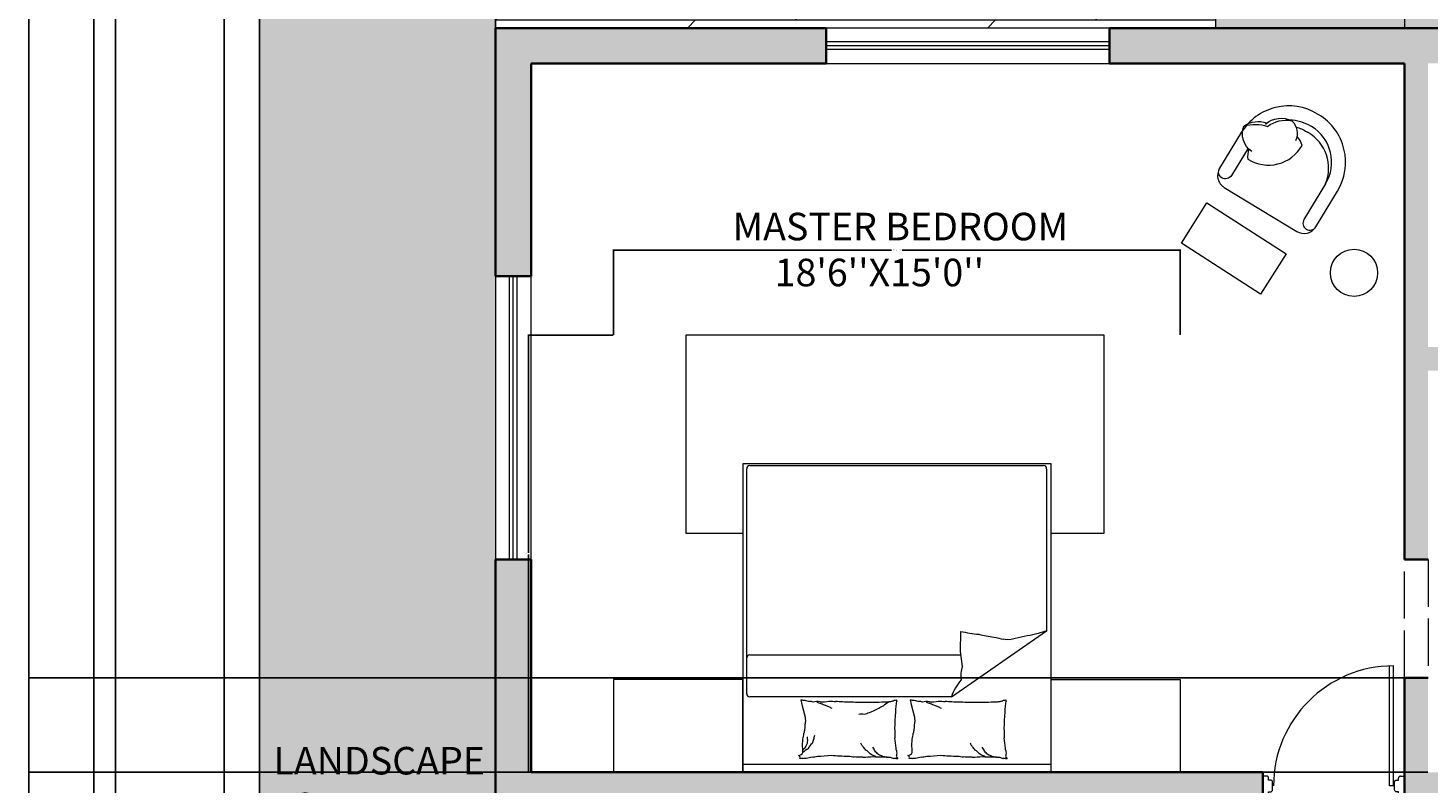
# Model space of a CAD drawing. Units: inches. Extents: x 84 to 1044, y -280 to 906.
# Tile 50 of 105: x 84 to 440, y 517 to 709. Entities that reach past the tile are written whole.
import ezdxf

# ---------------------------------------------------------------- set-up
doc = ezdxf.new("R2010")
doc.units = ezdxf.units.IN
doc.linetypes.add('ACAD_ISO02W100', pattern=[15, 12, -3])
for name, color, linetype, lineweight in [('00 FURNITURE', 15, 'Continuous', 15), ('A-ANNO-DIMS', 2, 'Continuous', 18), ('A-ANNO-TTLB', 7, 'Continuous', 25), ('A-AREA-IDEN', 7, 'Continuous', 13), ('A-DOOR', 4, 'Continuous', 18), ('A-FURN', 8, 'Continuous', 15), ('A-WALL-OVHD', 8, 'ACAD_ISO02W100', 13), ('C-PROP', 7, 'Continuous', 25), ('L-HRDS', 32, 'Continuous', 18), ('WALL', 250, 'Continuous', 35), ('WINDOW', 160, 'Continuous', 13)]:
    doc.layers.add(name, color=color, linetype=linetype, lineweight=lineweight)
for name, color, linetype, lineweight, true_color in [('A-FLOR-PATT', 251, 'Continuous', 9, 0x705861), ('A-WALL-PATT', 251, 'Continuous', 9, 0x636466), ('L-PLNT-PATT', 9, 'Continuous', 9, 0xafd9aa)]:
    doc.layers.add(name, color=color, linetype=linetype, lineweight=lineweight, true_color=true_color)
doc.styles.add('1-100DIM', font='txt', dxfattribs={"height": 0.3})
doc.styles.get("Standard").update_dxf_attribs({"font": 'arial.ttf'})
doc.dimstyles.get("Standard").update_dxf_attribs({"dimtxt": 0.18, "dimasz": 0.18, "dimexe": 0.18, "dimexo": 0.0625, "dimgap": 0.09, "dimtad": 0, "dimtih": 1, "dimtoh": 1, "dimdec": 4, "dimzin": 0, "dimdsep": 46, "dimtxsty": 'Standard', "dimcen": 0.09, "dimadec": 0, "dimazin": 0, "dimtfac": 1, "dimtdec": 4, "dimtofl": 0, "dimtmove": 0, "dimatfit": 3, "dimfxl": 1, "dimtolj": 1, "dimtzin": 0, "dimarcsym": 0})

# ---------------------------------------------------------------- blocks, each defined once
blk = doc.blocks.new('DDD')
at = {"layer": '00 FURNITURE'}
for p, q in [((-12579.77, -15859.53), (-12579.77, -15829.05)), ((-12578.77, -15859.53), (-12578.77, -15829.03)), ((-12612.02, -15857.03), (-12612.02, -15862.03)), ((-12611.02, -15857.03), (-12612.02, -15857.03)), ((-12577.02, -15857.03), (-12576.02, -15857.03)), ((-12576.02, -15857.03), (-12576.02, -15862.03)), ((-12610.52, -15858.03), (-12610.52, -15857.53)), ((-12578.77, -15859.53), (-12579.77, -15859.53)), ((-12577.52, -15858.03), (-12577.52, -15857.53)), ((-12612.02, -15862.03), (-12611.02, -15862.03)), ((-12610.52, -15861.53), (-12610.52, -15861.03)), ((-12577.52, -15861.53), (-12577.52, -15861.03)), ((-12576.02, -15862.03), (-12577.02, -15862.03))]:
    blk.add_line(p, q, dxfattribs=at)
for points in [[(-12610.52, -15861.03), (-12610.02, -15861.03, 0.414214), (-12609.52, -15860.53), (-12609.52, -15858.53, 0.414214), (-12610.02, -15858.03), (-12610.52, -15858.03)], [(-12577.52, -15861.03), (-12578.02, -15861.03, -0.414214), (-12578.52, -15860.53), (-12578.52, -15858.53, -0.414214), (-12578.02, -15858.03), (-12577.52, -15858.03)]]:
    blk.add_lwpolyline(points, format="xyb", dxfattribs=at)
for centre, radius, start, end in [((-12578.77, -15859.53), 30.5, 90, 180), ((-12611.02, -15857.53), 0.5, 0, 90), ((-12577.02, -15857.53), 0.5, 90, 180), ((-12611.02, -15861.53), 0.5, 270, 0), ((-12577.02, -15861.53), 0.5, 180, 270)]:
    blk.add_arc(centre, radius, start, end, dxfattribs=at)
blk = doc.blocks.new('BED-DOUBLE-NIGHTSTANDS')
for p, q in [((33.85, 19.92), (33.85, 77.08)), ((34.63, 77.86), (109.28, 77.86)), ((110.06, 77.08), (110.06, 35.88)), ((85.85, 19.14), (110.06, 35.88)), ((88.16, 30.61), (88.22, 35.71)), ((34.63, 29.81), (88.27, 29.81)), ((88.69, 26.88), (88.16, 30.61)), ((85.85, 19.14), (34.63, 19.14)), ((47.6, 18.34), (47.89, 17.17)), ((75.38, 18.34), (75.67, 17.17)), ((47.89, 17.17), (48.7, 13.93)), ((75.67, 17.17), (76.48, 13.93)), ((32.83, 2.05), (111.17, 2.05))]:
    blk.add_line(p, q)
blk.add_lwpolyline([(111.17, 60.71), (124.69, 60.71), (124.69, 111), (18.36, 111), (18.36, 60.71), (32.83, 60.71)])
for points in [[(32.83, 78.34), (32.83, 0), (111.17, 0), (111.17, 78.34)], [(0, 23.5), (0, 0), (32.83, 0), (32.83, 23.5)], [(144, 23.5), (144, 0), (111.17, 0), (111.17, 23.5)]]:
    blk.add_lwpolyline(points, close=True)
for centre, radius, start, end in [((34.63, 77.08), 0.783, 90, 180), ((109.28, 77.08), 0.783, 0, 90), ((112.65, 181.75), 148.07, 260.505, 262.308), ((129.8, -33.24), 71.88, 105.9352, 107.7364), ((113.34, 134.29), 101.37, 258.3259, 260.505), ((119.11, 130.25), 98.54, 256.8096, 258.3259), ((98.14, 26.21), 7.6, 76.8096, 82.2696), ((100.3, 31.38), 2.28, 82.2696, 100.7276), ((136.22, -121.54), 159.21, 100.7276, 102.9255), ((113.66, 10.12), 25.75, 102.9255, 105.9352), ((34.63, 29.03), 0.783, 90, 180), ((95.31, 24.45), 7.05, 159.8512, 188.1356), ((99.64, 14.08), 14.69, 140.3555, 159.8512), ((34.63, 19.92), 0.783, 180, 270), ((47.6, 18.38), 0.0359, 265.9171, 14.0449), ((49.38, 28.85), 10.61, 260.5159, 265.9171), ((51.31, 26.86), 9, 252.6136, 260.5159), ((49.31, 13.32), 4.69, 72.6136, 83.5659), ((51.85, 12.2), 5.72, 83.5659, 101.5586), ((52.93, 26.88), 9.01, 267.2509, 281.5586), ((59.16, 72.9), 55.02, 265.3824, 267.2509), ((54.35, -29.66), 47.65, 85.3824, 87.3904), ((55.96, -113.85), 131.7, 87.3904, 89.0296), ((85.21, -6.34), 28.54, 122.135, 125.8263), ((70.75, 12.2), 5.71, 93.574, 102.869), ((71.21, 16.33), 1.77, 102.869, 117.2841), ((69.98, 20.94), 3.01, 286.2212, 297.2841), ((70.93, 21.67), 3.43, 277.1204, 286.2212), ((59.41, 18.76), 12.58, 350.0016, 356.4951), ((71.94, 18.4), 0.0517, 196.6978, 277.1204), ((72.69, 18.21), 0.757, 170.0016, 196.6978), ((75.38, 18.38), 0.0359, 265.9171, 14.0449), ((77.16, 28.85), 10.61, 260.5159, 265.9171), ((79.09, 26.86), 9, 252.6136, 260.5159), ((77.09, 13.32), 4.69, 72.6136, 83.5659), ((79.63, 12.2), 5.72, 83.5659, 101.5586), ((80.71, 26.88), 9.01, 267.2509, 281.5586), ((86.94, 72.9), 55.02, 265.3824, 267.2509), ((82.13, -29.66), 47.65, 85.3824, 87.3904), ((83.74, -113.85), 131.7, 87.3904, 89.0296), ((98.54, 12.2), 5.71, 93.574, 102.869), ((98.99, 16.33), 1.77, 102.869, 117.2841), ((97.76, 20.94), 3.01, 286.2212, 297.2841), ((98.71, 21.67), 3.43, 277.1204, 286.2212), ((87.19, 18.76), 12.58, 350.0016, 356.4951), ((99.72, 18.4), 0.0517, 196.6978, 277.1204), ((100.47, 18.21), 0.757, 170.0016, 196.6978), ((61.28, 45.06), 28.93, 250.572, 252.8018), ((63.4, 44.31), 28.93, 248.3423, 250.572), ((65.3, 43.56), 28.93, 246.5156, 248.3423), ((67, 42.82), 28.93, 244.6889, 246.5156), ((63.07, -206.28), 223.99, 89.0296, 90.2865), ((63.07, 4.04), 10.66, 86.4448, 94.0828), ((64.53, 12.55), 2.27, 94.0828, 110.6743), ((72.54, -3.27), 19.85, 110.6743, 114.3265), ((90.57, -34.91), 56.1, 114.3265, 116.4985), ((69.71, -27.82), 45.59, 90.2865, 93.574), ((73.97, 5.84), 12.25, 116.4985, 122.135), ((-461.55, 45.04), 534.1, 356.4951, 356.945), ((89.06, 45.06), 28.93, 250.572, 252.8018), ((91.18, 44.31), 28.93, 248.3423, 250.572), ((93.09, 43.56), 28.93, 246.5156, 248.3423), ((94.78, 42.82), 28.93, 244.6889, 246.5156), ((90.85, -206.28), 223.99, 89.0296, 90.2865), ((97.49, -27.82), 45.59, 90.2865, 93.574), ((-433.77, 45.04), 534.1, 356.4951, 356.945), ((60.69, 8.15), 12.42, 167.8016, 171.9949), ((74.33, 9.57), 25.8, 171.9949, 177.3351), ((51.35, 13.81), 2.65, 177.3351, 194.0452), ((18.1, 13.92), 53.48, 356.945, 358.3669), ((44.96, 9.51), 26.59, 358.3669, 3.3687), ((88.47, 8.15), 12.42, 167.8016, 171.9949), ((102.11, 9.57), 25.8, 171.9949, 177.3351), ((79.13, 13.81), 2.65, 177.3351, 194.0452), ((45.88, 13.92), 53.48, 356.945, 358.3669), ((72.74, 9.51), 26.59, 358.3669, 3.3687), ((40.12, 8.39), 7.99, 350.3156, 0), ((14.34, 15.69), 34.55, 347.8016, 350.3156), ((56.69, 4.33), 8.05, 158.1851, 161.2201), ((52.8, 8.94), 3.59, 180, 194.6851), ((51.41, 7.32), 2.2, 161.2201, 180), ((54.33, 3.44), 5.48, 134.9024, 152.6012), ((55.72, 5.76), 5.48, 152.6012, 163.485), ((56.31, 7.75), 5.48, 163.485, 174.3689), ((55.99, 3.67), 7.84, 23.0028, 28.3168), ((36.09, 3.97), 35.76, 3.3687, 7.6809), ((67.9, 8.39), 7.99, 350.3156, 0), ((42.12, 15.69), 34.55, 347.8016, 350.3156), ((83.77, 3.67), 7.84, 23.0028, 28.3168), ((63.87, 3.97), 35.76, 3.3687, 7.6809), ((46.91, 5.57), 1.34, 274.4002, 333.4195), ((46.92, 3.73), 0.514, 333.4195, 78.7276), ((28.84, 4.95), 19.27, 0, 6.2324), ((50.68, 3.26), 3.52, 126.2641, 138.5571), ((51.97, 1.08), 5.48, 117.2036, 134.9024), ((50.46, 5.22), 2.06, 138.5571, 154.6449), ((54.41, 4.38), 5.92, 154.6449, 158.1851), ((52.23, -7.99), 11.94, 98.4372, 105.744), ((49.23, 13.22), 9.49, 277.5469, 285.744), ((51.81, 30.83), 26.74, 270, 277.5469), ((59.68, 45.18), 41.09, 263.9133, 270), ((63.35, 24.49), 20.73, 259.8101, 263.9133), ((60.88, -2.08), 5.97, 79.8101, 87.4614), ((62.89, -7.52), 11.35, 87.4614, 94.8018), ((61.71, 5.52), 1.93, 28.3168, 39.0349), ((63.05, 38.02), 34.2, 270.5757, 274.8018), ((57.3, 0.07), 8.82, 39.0349, 46.1885), ((54.63, -6.4), 15.34, 46.1885, 51.6114), ((63.87, 2), 3.01, 51.6114, 62.7604), ((62.48, -4.21), 9.17, 62.7604, 69.1397), ((62.77, 4.07), 3.89, 18.4397, 36.1766), ((67.86, 62.44), 58.53, 268.0921, 270.5757), ((64.17, 2.16), 3.89, 36.1766, 53.9136), ((66.24, 0.72), 3.89, 53.9136, 74.0648), ((71.39, 35.92), 32.15, 264.7408, 268.0921), ((68.82, -0.02), 3.89, 74.0648, 94.2159), ((71.4, 5.61), 2.11, 239.3487, 264.7408), ((64.2, 4.44), 7.77, 7.6809, 12.1095), ((81.44, 6.84), 9.64, 188.1335, 192.1095), ((73.21, 4.35), 1.28, 158.579, 188.1335), ((71.37, 3.94), 0.611, 338.579, 21.9904), ((71.98, 3.55), 0.168, 21.9904, 101.8931), ((72.22, 3.59), 0.0908, 160.436, 281.8931), ((74.69, 5.57), 1.34, 274.4002, 333.4195), ((74.7, 3.73), 0.514, 333.4195, 78.7276), ((56.62, 4.95), 19.27, 0, 6.2324), ((80.01, -7.99), 11.94, 98.4372, 105.744), ((77.02, 13.22), 9.49, 277.5469, 285.744), ((79.59, 30.83), 26.74, 270, 277.5469), ((87.46, 45.18), 41.09, 263.9133, 270), ((91.13, 24.49), 20.73, 259.8101, 263.9133), ((88.66, -2.08), 5.97, 79.8101, 87.4614), ((90.67, -7.52), 11.35, 87.4614, 94.8018), ((89.49, 5.52), 1.93, 28.3168, 39.0349), ((90.83, 38.02), 34.2, 270.5757, 274.8018), ((85.08, 0.07), 8.82, 39.0349, 46.1885), ((82.41, -6.4), 15.34, 46.1885, 51.6114), ((91.65, 2), 3.01, 51.6114, 62.7604), ((90.26, -4.21), 9.17, 62.7604, 69.1397), ((90.56, 4.07), 3.89, 18.4397, 36.1766), ((95.64, 62.44), 58.53, 268.0921, 270.5757), ((91.95, 2.16), 3.89, 36.1766, 53.9136), ((94.02, 0.72), 3.89, 53.9136, 74.0648), ((99.18, 35.92), 32.15, 264.7408, 268.0921), ((96.6, -0.02), 3.89, 74.0648, 94.2159), ((99.18, 5.61), 2.11, 239.3487, 264.7408), ((91.98, 4.44), 7.77, 7.6809, 12.1095), ((109.22, 6.84), 9.64, 188.1335, 192.1095), ((100.99, 4.35), 1.28, 158.579, 188.1335), ((99.15, 3.94), 0.611, 338.579, 21.9904), ((99.76, 3.55), 0.168, 21.9904, 101.8931), ((100, 3.59), 0.0908, 160.436, 281.8931), ((47.38, -0.04), 3.54, 78.7276, 90), ((48.99, -2.82), 6.31, 90, 98.4372), ((71.29, 2.38), 1.13, 59.3487, 94.3025), ((72.23, 2.44), 0.984, 94.3025, 111.7883), ((72.29, 3.37), 0.134, 111.7883, 160.436), ((75.16, -0.04), 3.54, 78.7276, 90), ((76.77, -2.82), 6.31, 90, 98.4372), ((99.07, 2.38), 1.13, 59.3487, 94.3025), ((100.02, 2.44), 0.984, 94.3025, 111.7883), ((100.07, 3.37), 0.134, 111.7883, 160.436)]:
    blk.add_arc(centre, radius, start, end)
blk = doc.blocks.new('CHAIR-LOUNGE')
for points in [[(10.9, 6.11), (20.11, 0.51, 0.414214), (24.96, 1.7), (30.46, 10.75, 0.414214), (25.72, 30.16), (25.57, 30.25), (25.42, 30.34, 0.414214), (6.01, 25.61), (0.51, 16.55, 0.414214), (1.69, 11.7), (10.9, 6.11)], [(6.69, 27.28, -0.14773), (12.68, 27.2, -0.213343), (18.88, 28.63, -0.178662)], [(12.19, 27.77, -0.306663), (18.88, 28.63, -0.30633), (19.83, 23.56, 0.872847)], [(18.37, 28.86, -0.130591), (23.59, 27.33), (23.74, 27.24)], [(8.7, 20.85, -0.356772), (6.69, 27.28, -0.249542), (12.51, 28.04, 9.61688)], [(19.9, 27.06, -0.072384), (22.67, 25.82), (22.82, 25.73)], [(27.44, 12.59, 0.372719), (22.97, 25.63), (22.82, 25.73)], [(27.44, 12.59, 0.414214), (23.89, 27.14), (23.74, 27.24)], [(7.74, 21.66), (3.53, 14.72, -0.414214), (1.1, 14.13), (1.1, 14.13, -0.414214), (0.51, 16.55)], [(8, 21.4, 0.165541), (7.72, 18.84, 0.425989), (21.45, 22.34, 0.121523), (20.16, 24.75, -7.115464)], [(27.44, 12.59), (21.94, 3.53, 0.414214), (22.53, 1.11), (22.53, 1.11, 0.414214), (24.96, 1.7)]]:
    blk.add_lwpolyline(points, format="xyb")
blk = doc.blocks.new('WIN-72IN')
for p, q in [((72, 9), (0, 9)), ((72, 5.5), (0, 5.5)), ((72, 4.5), (0, 4.5)), ((72, 3.5), (0, 3.5)), ((0, 0), (72, 0))]:
    blk.add_line(p, q)
blk = doc.blocks.new('*D50')
at = {"layer": 'A-ANNO-DIMS', "color": 0, "lineweight": -2, "transparency": 16777216}
for p, q in [((233.13, 631.18), (233.13, 652.9)), ((233.31, 652.72), (303.74, 652.72)), ((376.95, 652.72), (306.51, 652.72)), ((377.13, 631.18), (377.13, 652.9))]:
    blk.add_line(p, q, dxfattribs=at)
at = {"layer": 'A-ANNO-DIMS', "color": 0, "transparency": 16777216}
for points in [[(233.31, 652.75), (233.31, 652.69), (233.13, 652.72)], [(376.95, 652.75), (376.95, 652.69), (377.13, 652.72)]]:
    blk.add_solid(points, dxfattribs=at)
at = {"layer": 'Defpoints', "color": 0, "transparency": 16777216}
for p in [(377.13, 652.72), (233.13, 631.12), (377.13, 631.12)]:
    blk.add_point(p, dxfattribs=at)
at = {"layer": 'A-ANNO-DIMS', "color": 0, "transparency": 16777216, "insert": (305.13, 652.72), "char_height": 0.18, "attachment_point": 5}
blk.add_mtext('\\A1;BED GROUP 144 TYP.', dxfattribs=at)
blk = doc.blocks.new('*D51')
at = {"layer": 'A-ANNO-DIMS', "color": 0, "lineweight": -2, "transparency": 16777216}
for p, q in [((233.06, 631.12), (211.35, 631.12)), ((211.53, 630.94), (211.53, 575.8)), ((211.53, 520.3), (211.53, 575.44)), ((233.06, 520.12), (211.35, 520.12))]:
    blk.add_line(p, q, dxfattribs=at)
at = {"layer": 'A-ANNO-DIMS', "color": 0, "transparency": 16777216}
for points in [[(211.5, 630.94), (211.56, 630.94), (211.53, 631.12)], [(211.5, 520.3), (211.56, 520.3), (211.53, 520.12)]]:
    blk.add_solid(points, dxfattribs=at)
at = {"layer": 'Defpoints', "color": 0, "transparency": 16777216}
for p in [(211.53, 631.12), (233.13, 631.12), (233.13, 520.12)]:
    blk.add_point(p, dxfattribs=at)
at = {"layer": 'A-ANNO-DIMS', "color": 0, "transparency": 16777216, "insert": (211.53, 575.62), "char_height": 0.18, "attachment_point": 5}
blk.add_mtext('\\A1;111 TYP.', dxfattribs=at)
blk = doc.blocks.new('*D61')
at = {"layer": 'A-ANNO-DIMS', "color": 0, "lineweight": -2, "transparency": 16777216}
for p, q in [((134.12, 856.12), (84.4, 856.12)), ((84.58, 855.94), (84.58, 367.3)), ((84.58, -121.7), (84.58, 366.94)), ((134.12, -121.88), (84.4, -121.88))]:
    blk.add_line(p, q, dxfattribs=at)
at = {"layer": 'A-ANNO-DIMS', "color": 0, "transparency": 16777216}
for points in [[(84.55, 855.94), (84.61, 855.94), (84.58, 856.12)], [(84.55, -121.7), (84.61, -121.7), (84.58, -121.88)]]:
    blk.add_solid(points, dxfattribs=at)
at = {"layer": 'Defpoints', "color": 0, "transparency": 16777216}
for p in [(84.58, 856.12), (134.18, 856.12), (134.18, -121.88)]:
    blk.add_point(p, dxfattribs=at)
at = {"layer": 'A-ANNO-DIMS', "color": 0, "transparency": 16777216, "insert": (84.58, 367.12), "char_height": 0.18, "attachment_point": 5}
blk.add_mtext('\\A1;978', dxfattribs=at)
blk = doc.blocks.new('*D62')
at = {"layer": 'A-ANNO-DIMS', "color": 0, "lineweight": -2, "transparency": 16777216}
for p, q in [((203.18, 709.18), (203.18, 905.9)), ((203.36, 905.72), (549.23, 905.72)), ((895.89, 905.72), (550.02, 905.72)), ((896.07, 400.18), (896.07, 905.9))]:
    blk.add_line(p, q, dxfattribs=at)
at = {"layer": 'A-ANNO-DIMS', "color": 0, "transparency": 16777216}
for points in [[(203.36, 905.75), (203.36, 905.69), (203.18, 905.72)], [(895.89, 905.75), (895.89, 905.69), (896.07, 905.72)]]:
    blk.add_solid(points, dxfattribs=at)
at = {"layer": 'Defpoints', "color": 0, "transparency": 16777216}
for p in [(896.07, 905.72), (203.18, 709.12), (896.07, 400.12)]:
    blk.add_point(p, dxfattribs=at)
at = {"layer": 'A-ANNO-DIMS', "color": 0, "transparency": 16777216, "insert": (549.63, 905.72), "char_height": 0.18, "attachment_point": 5}
blk.add_mtext('\\A1;692.9', dxfattribs=at)
blk = doc.blocks.new('*D74')
at = {"layer": 'A-ANNO-DIMS', "color": 0, "lineweight": -2, "transparency": 16777216}
for p, q in [((440.01, 544.12), (84.4, 544.12)), ((84.58, 543.94), (84.58, 532.3)), ((84.58, 520.3), (84.58, 531.94)), ((440.01, 520.12), (84.4, 520.12))]:
    blk.add_line(p, q, dxfattribs=at)
at = {"layer": 'A-ANNO-DIMS', "color": 0, "transparency": 16777216}
for points in [[(84.55, 543.94), (84.61, 543.94), (84.58, 544.12)], [(84.55, 520.3), (84.61, 520.3), (84.58, 520.12)]]:
    blk.add_solid(points, dxfattribs=at)
at = {"layer": 'Defpoints', "color": 0, "transparency": 16777216}
for p in [(84.58, 544.12), (440.07, 544.12), (440.07, 520.12)]:
    blk.add_point(p, dxfattribs=at)
at = {"layer": 'A-ANNO-DIMS', "color": 0, "transparency": 16777216, "insert": (84.58, 532.12), "char_height": 0.18, "attachment_point": 5}
blk.add_mtext('\\A1;24', dxfattribs=at)

msp = doc.modelspace()

# ---------------------------------------------------------------- hatches: boundary and pattern name
at = {"layer": 'A-FLOR-PATT', "transparency": 33554597}
h = msp.add_hatch(dxfattribs=at)
h.set_pattern_fill('DOLMIT', color=256)
h.paths.add_polyline_path([(896.074, 709.12), (833.074, 709.12), (833.074, 646.12), (833.074, 574.12), (833.074, 511.12), (896.074, 511.12)])
h.paths.add_polyline_path([(386.074, 769.12), (203.179, 769.12), (203.179, 709.12), (287.127, 709.12), (359.127, 709.12), (386.074, 709.12)])
at = {"layer": 'A-WALL-PATT', "transparency": 33554597}
h = msp.add_hatch(color=256, dxfattribs=at)
h.dxf.hatch_style = 1
h.paths.add_polyline_path([(671.074, 100.12), (647.074, 100.12), (647.074, 160.12), (641.074, 160.12), (620.824, 160.12), (620.824, 151.12), (638.074, 151.12), (638.074, 91.12), (671.074, 91.12)])
h.paths.add_polyline_path([(791.074, 100.12), (743.074, 100.12), (743.074, 91.12), (791.074, 91.12)])
h.paths.add_polyline_path([(896.074, 346.12), (887.074, 346.12), (887.074, 334.12), (870.955, 334.12), (833.074, 334.12), (804.574, 334.12), (804.574, 328.12), (887.074, 328.12), (887.074, 100.12), (863.074, 100.12), (863.074, 91.12), (896.074, 91.12)])
h.paths.add_polyline_path([(507.574, 154.729), (507.574, 160.12), (464.074, 160.12), (464.074, 247.12), (641.074, 247.12), (641.074, 208.12), (647.074, 208.12), (647.074, 328.12), (659.074, 328.12), (659.074, 334.12), (617.074, 334.12), (617.074, 328.12), (641.074, 328.12), (641.074, 256.12), (545.074, 256.12), (545.074, 328.12), (569.074, 328.12), (569.074, 334.12), (518.074, 334.12), (518.074, 325.12), (536.074, 325.12), (536.074, 256.12), (464.074, 256.12), (464.074, 325.12), (482.074, 325.12), (482.074, 334.12), (455.074, 334.12), (455.074, 160.12), (413.127, 160.12), (413.127, 151.12), (455.074, 151.12), (455.074, 91.12), (464.074, 91.12), (464.074, 151.12), (507.574, 151.12)])
h.paths.add_polyline_path([(572.824, 160.12), (555.574, 160.12), (555.574, 151.12), (572.824, 151.12)], flags=17)
h.paths.add_polyline_path([(341.127, 160.12), (299.179, 160.12), (299.179, 211.12), (294.179, 211.12), (290.179, 211.12), (290.179, 151.12), (341.127, 151.12)])
h.paths.add_polyline_path([(299.179, 256.12), (212.179, 256.12), (212.179, 274.12), (203.179, 274.12), (203.179, 247.12), (299.179, 247.12)])
h.paths.add_polyline_path([(212.179, 514.12), (398.074, 514.12), (398.074, 519.12), (398.074, 520.12), (212.179, 520.12), (212.179, 574.12), (203.179, 574.12), (203.179, 310.12), (212.179, 310.12), (212.179, 328.12), (290.179, 328.12), (290.179, 292.12), (299.179, 292.12), (299.179, 328.12), (332.179, 328.12), (332.179, 334.12), (212.179, 334.12)])
h.paths.add_polyline_path([(287.127, 709.12), (203.179, 709.12), (203.179, 646.12), (212.179, 646.12), (212.179, 700.12), (287.127, 700.12)])
h.paths.add_polyline_path([(470.074, 709.12), (359.127, 709.12), (359.127, 700.12), (434.074, 700.12), (434.074, 574.12), (440.074, 574.12), (440.074, 622.12), (464.074, 622.12), (464.074, 628.12), (440.074, 628.12), (440.074, 700.12), (470.074, 700.12)])
h.paths.add_polyline_path([(572.074, 709.12), (506.074, 709.12), (506.074, 700.12), (536.074, 700.12), (536.074, 628.12), (494.074, 628.12), (494.074, 622.12), (536.074, 622.12), (536.074, 520.12), (440.074, 520.12), (440.074, 544.12), (434.074, 544.12), (434.074, 514.12), (644.074, 514.12), (644.074, 519.12), (644.074, 544.12), (638.074, 544.12), (638.074, 520.12), (542.074, 520.12), (542.074, 622.12), (584.074, 622.12), (584.074, 628.12), (542.074, 628.12), (542.074, 700.12), (572.074, 700.12)])
h.paths.add_polyline_path([(698.074, 709.12), (608.074, 709.12), (608.074, 700.12), (638.074, 700.12), (638.074, 628.12), (614.074, 628.12), (614.074, 622.12), (638.074, 622.12), (638.074, 574.12), (644.074, 574.12), (644.074, 700.12), (698.074, 700.12)])
h.paths.add_polyline_path([(833.074, 709.12), (770.074, 709.12), (770.074, 700.12), (824.074, 700.12), (824.074, 646.12), (833.074, 646.12)])
h.paths.add_polyline_path([(833.074, 574.12), (824.074, 574.12), (824.074, 520.12), (791.244, 520.12), (712.904, 520.12), (680.074, 520.12), (680.074, 514.12), (695.074, 514.12), (695.074, 491.62), (704.074, 491.62), (704.074, 511.12), (833.074, 511.12)])
h.paths.add_polyline_path([(704.074, 419.62), (695.074, 419.62), (695.074, 370.12), (704.074, 370.12)])
h.paths.add_polyline_path([(896.074, 400.12), (833.074, 400.12), (833.074, 364.12), (839.074, 364.12), (839.074, 394.12), (887.074, 394.12), (887.074, 382.12), (896.074, 382.12)])
h.paths.add_polyline_path([(732.574, 334.12), (695.074, 334.12), (695.074, 328.12), (732.574, 328.12)])
at = {"layer": 'L-PLNT-PATT', "transparency": 33554597}
h = msp.add_hatch(color=256, dxfattribs=at)
h.dxf.hatch_style = 1
h.paths.add_polyline_path([(434.074, 769.12), (386.074, 769.12), (386.074, 709.12), (434.074, 709.12)])
h.paths.add_polyline_path([(896.074, 847.12), (434.074, 847.12), (434.074, 769.12), (434.074, 709.12), (470.074, 709.12), (506.074, 709.12), (572.074, 709.12), (608.074, 709.12), (698.074, 709.12), (770.074, 709.12), (833.074, 709.12), (896.074, 709.12)])
h.paths.add_polyline_path([(983.074, 847.12), (896.074, 847.12), (896.074, 709.12), (896.074, 547.12), (932.074, 547.12), (983.074, 547.12)])
h.paths.add_polyline_path([(983.074, 547.12), (932.074, 547.12), (932.074, 265.12), (983.074, 265.12)])
h.paths.add_polyline_path([(203.179, 646.12), (203.179, 709.12), (203.179, 745.12), (143.179, 745.12), (143.179, 271.12), (203.179, 271.12), (203.179, 274.12), (203.179, 310.12), (203.179, 574.12)])

# ---------------------------------------------------------------- linework, layer by layer
at = {"layer": 'A-ANNO-TTLB'}
for points in [[(101.1, 905.916), (1027.308, 905.916), (1027.308, -279.764), (101.1, -279.764)], [(106.576, 900.439), (1021.832, 900.439), (1021.832, -274.288), (106.576, -274.288)]]:
    msp.add_lwpolyline(points, close=True, dxfattribs=at)
at = {"layer": 'A-FURN'}
msp.add_lwpolyline([(404.08, 651.779), (397.515, 641.562), (377.475, 654.437), (383.888, 664.752)], close=True, dxfattribs=at)
msp.add_circle((421.278, 646.943), 6, dxfattribs=at)
at = {"layer": 'A-WALL-OVHD'}
msp.add_lwpolyline([(434.074, 574.12), (440.074, 574.12), (440.074, 544.12), (434.074, 544.12)], close=True, dxfattribs=at)
at = {"layer": 'C-PROP'}
for points in [[(143.179, -121.88), (134.179, -121.88), (134.179, 856.12), (992.074, 856.12), (992.074, -121.88), (624.574, -121.88)], [(143.179, -112.88), (143.179, 847.12), (983.074, 847.12), (983.074, -112.88), (624.574, -112.88)]]:
    msp.add_lwpolyline(points, dxfattribs=at)
at = {"layer": 'L-HRDS'}
for p, q in [((203.179, 709.12), (203.179, 769.12)), ((386.074, 769.12), (386.074, 709.12)), ((434.074, 769.12), (434.074, 709.12))]:
    msp.add_line(p, q, dxfattribs=at)
at = {"layer": 'WALL'}
for p, q in [((203.179, 709.12), (203.179, 646.12)), ((287.127, 709.12), (203.179, 709.12)), ((287.127, 700.12), (287.127, 709.12)), ((359.127, 700.12), (359.127, 709.12)), ((470.074, 709.12), (359.127, 709.12)), ((287.127, 700.12), (212.179, 700.12)), ((212.179, 646.12), (212.179, 700.12)), ((434.074, 700.12), (359.127, 700.12)), ((434.074, 574.12), (434.074, 700.12)), ((212.179, 646.12), (203.179, 646.12)), ((212.179, 574.12), (203.179, 574.12)), ((203.179, 574.12), (203.179, 310.12)), ((212.179, 520.12), (212.179, 574.12)), ((440.074, 574.12), (434.074, 574.12)), ((434.074, 514.12), (434.074, 544.12)), ((440.074, 544.12), (434.074, 544.12)), ((398.074, 520.12), (212.179, 520.12)), ((398.074, 514.12), (398.074, 520.12))]:
    msp.add_line(p, q, dxfattribs=at)

# ---------------------------------------------------------------- block references
at = {"layer": 'A-DOOR'}
msp.add_blockref('DDD', (13010.097, 16376.149), dxfattribs=at)
at = {"layer": 'A-FURN'}
for name, p in [('CHAIR-LOUNGE', (386.62, 656.94)), ('BED-DOUBLE-NIGHTSTANDS', (233.123, 520.12))]:
    msp.add_blockref(name, p, dxfattribs=at)
at = {"layer": 'WINDOW'}
msp.add_blockref('WIN-72IN', (287.123, 700.12), dxfattribs=at)
at = {"layer": 'WINDOW', "rotation": 269.9999999999999}
msp.add_blockref('WIN-72IN', (203.179, 646.124), dxfattribs=at)

# ---------------------------------------------------------------- texts
at = {"layer": 'A-AREA-IDEN', "char_height": 7, "attachment_point": 1, "style": '1-100DIM'}
for s, width, insert in [("{\\f@Malgun Gothic|b0|i0|c0|p34;MASTER BEDROOM\\P     18'6''X15'0''}", 94.39973, (263.392, 662.194)), ('{\\f@Malgun Gothic|b0|i0|c0|p34;LANDSCAPE\\P  GARDEN}', 58.97918, (146.749, 526.534))]:
    msp.add_mtext_dynamic_manual_height_columns(s, width=width, gutter_width=15.851, heights=[0], dxfattribs=dict(at, insert=insert))

# ---------------------------------------------------------------- dimensions: what is measured, and where the dimension line sits
at = {"layer": 'A-ANNO-DIMS'}
dim = msp.add_linear_dim(base=(896.074, 905.72), p1=(203.179, 709.12), p2=(896.074, 400.12), dimstyle='Standard', override={"dimdec": 1, "dimlfac": 1, "dimrnd": 0, "dimzin": 0, "dimdsep": 46, "dimlunit": 2}, dxfattribs=at)
dim.commit()
dim.dimension.update_dxf_attribs({"geometry": '*D62', "text_midpoint": (549.627, 905.72)})
for base, p1, p2, picture, middle in [((84.579, 856.12), (134.179, -121.88), (134.179, 856.12), '*D61', (84.579, 367.12)), ((84.579, 544.12), (440.074, 520.12), (440.074, 544.12), '*D74', (84.579, 532.12))]:
    dim = msp.add_linear_dim(base=base, p1=p1, p2=p2, angle=90, dimstyle='Standard', override={"dimdec": 0, "dimlfac": 1, "dimrnd": 0, "dimzin": 0, "dimdsep": 46, "dimlunit": 2}, dxfattribs=at)
    dim.commit()
    dim.dimension.update_dxf_attribs({"geometry": picture, "text_midpoint": middle})
dim = msp.add_linear_dim(base=(377.127, 652.718), p1=(233.127, 631.118), p2=(377.127, 631.118), text='BED GROUP <> TYP.', dimstyle='Standard', override={"dimdec": 0, "dimlfac": 1, "dimrnd": 0, "dimzin": 0, "dimdsep": 46, "dimlunit": 2}, dxfattribs=at)
dim.commit()
dim.dimension.update_dxf_attribs({"geometry": '*D50', "text_midpoint": (305.127, 652.718)})
dim = msp.add_linear_dim(base=(211.527, 631.118), p1=(233.127, 520.12), p2=(233.127, 631.118), angle=90, text='<> TYP.', dimstyle='Standard', override={"dimdec": 0, "dimlfac": 1, "dimrnd": 0, "dimzin": 0, "dimdsep": 46, "dimlunit": 2}, dxfattribs=at)
dim.commit()
dim.dimension.update_dxf_attribs({"geometry": '*D51', "text_midpoint": (211.527, 575.619)})

doc.saveas('drawing.dxf')
